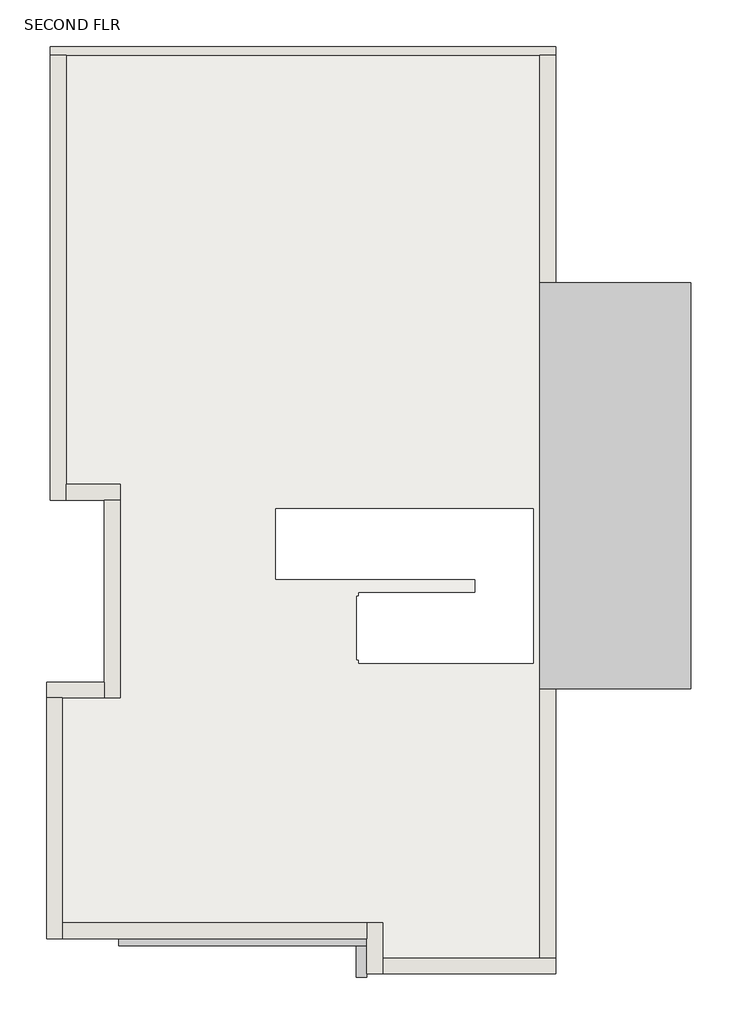
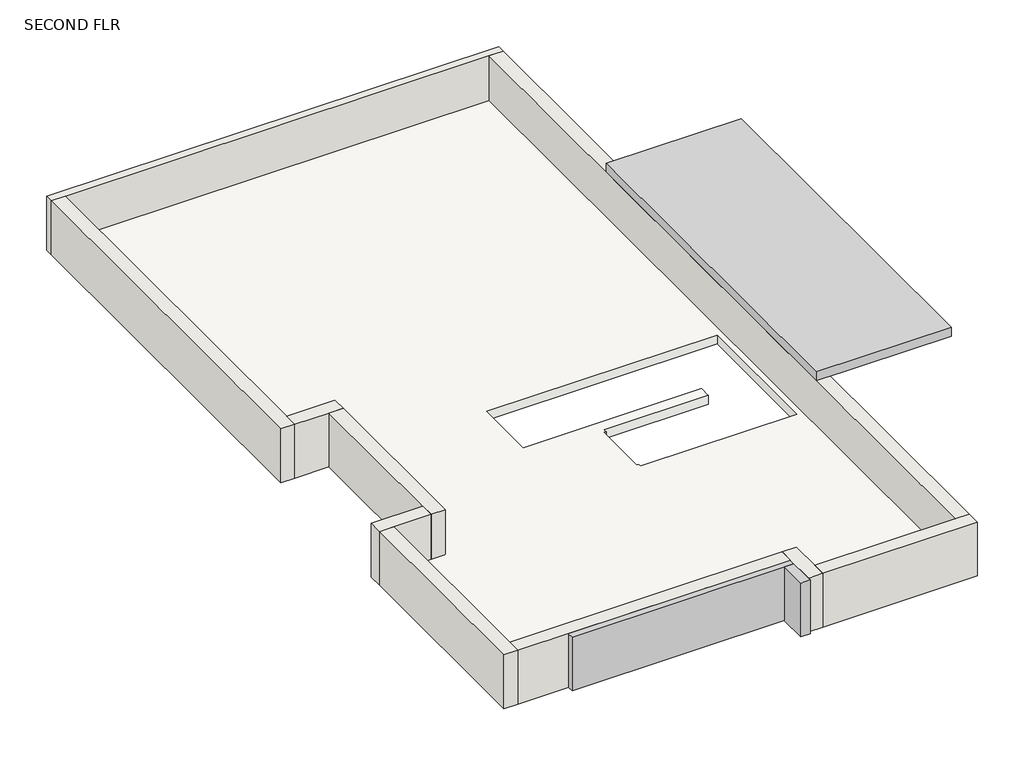
# One storey: 10 walls, 3 proxies, 1 roof.
"""IFC4 building model written with IfcOpenShell, lengths in millimetres."""

from ifc_helpers import new_model, si_unit, frame, origin, place, context, project, spatial, polyline, outline, extrude, faceted_brep, transform, mapped, element, save
from components import generic_models_10_generic_models_10_3c4deb4f, generic_models_4_generic_models_4_98a53d0d, generic_models_9_generic_models_9_5a9dd815

model = new_model("IFC4")

# Units and contexts
model_context = context("Model", 3, world=origin())
ifc_project = project(units=[si_unit("LENGTHUNIT", "METRE", prefix="MILLI")], contexts=[model_context])

# Site, building, storey
site = spatial("IfcSite", under=ifc_project)
building = spatial("IfcBuilding", under=site)
storey = spatial("IfcBuildingStorey", under=building, Name="SECOND FLR", Elevation=6096.0)

# Proxies
placement = place(None, origin())
generic_models_10_generic_models_10_shape = generic_models_10_generic_models_10_3c4deb4f(model_context)
element("IfcBuildingElementProxy", 1, Name="Generic Models 10 : Generic Models 10", ObjectType="Generic Models 10 : Generic Models 10", at=placement, inside=storey, context=model_context, shape_type="MappedRepresentation", body=[
    mapped(generic_models_10_generic_models_10_shape, transform((0.0, 0.0, 0.0), x_axis=(1.0, 0.0, 0.0), y_axis=(0.0, 1.0, 0.0), z_axis=(0.0, 0.0, 1.0))),
])
generic_models_4_generic_models_4_shape = generic_models_4_generic_models_4_98a53d0d(model_context)
element("IfcBuildingElementProxy", 2, Name="Generic Models 4 : Generic Models 4", ObjectType="Generic Models 4 : Generic Models 4", at=placement, inside=storey, context=model_context, shape_type="MappedRepresentation", body=[
    mapped(generic_models_4_generic_models_4_shape, transform((0.0, 0.0, 0.0), x_axis=(1.0, 0.0, 0.0), y_axis=(0.0, 1.0, 0.0), z_axis=(0.0, 0.0, 1.0))),
])
generic_models_9_generic_models_9_shape = generic_models_9_generic_models_9_5a9dd815(model_context)
element("IfcBuildingElementProxy", 3, Name="Generic Models 9 : Generic Models 9", ObjectType="Generic Models 9 : Generic Models 9", at=placement, inside=storey, context=model_context, shape_type="MappedRepresentation", body=[
    mapped(generic_models_9_generic_models_9_shape, transform((0.0, 0.0, 0.0), x_axis=(1.0, 0.0, 0.0), y_axis=(0.0, 1.0, 0.0), z_axis=(0.0, 0.0, 1.0))),
])

# Roof
element("IfcRoof", 4, ObjectType="FLOORING ROOF 6\"", at=placement, inside=storey, context=model_context, shape_type="SweptSolid", body=[
    extrude(outline(polyline([(-5910.1906521, 1140.4983389), (-5910.1906521, -11847.6453012), (-8170.7906521, -11847.6453012), (-8170.7906521, -11339.6453012), (-12780.8906521, -11339.6453012), (-12780.8906521, -8105.9310793), (-11952.140556, -8105.9310793), (-11952.140556, -5031.7016611), (-12726.840556, -5031.7016611), (-12726.840556, 1140.4983389), (-5910.1906521, 1140.4983389)]), holes=[polyline([(-8549.4760609, -7553.4810793), (-8517.7260609, -7553.4810793), (-8517.7260609, -7604.2810793), (-6003.1260609, -7604.2810793), (-6003.1260609, -5382.5504041), (-9709.3703437, -5382.5504041), (-9709.3703437, -6398.5504041), (-6841.3260609, -6398.5504041), (-6841.3260609, -6588.2810793), (-8517.7260609, -6588.2810793), (-8517.7260609, -6639.0810793), (-8549.4760609, -6639.0810793), (-8549.4760609, -7553.4810793)])]), frame((0.0, 0.0, 6096.0), z_axis=(0.0, 0.0, 1.0), x_axis=(1.0, 0.0, 0.0)), (0.0, 0.0, 1.0), 152.4),
])

# Walls
element("IfcWall", 5, ObjectType="EXTERIOR WALL 9\"", at=placement, inside=storey, context=model_context, shape_type="Brep", body=[
    faceted_brep([(-12955.440556, 1140.4983389, 6096.0), (-12955.440556, -5260.3016611, 6096.0), (-12955.440556, -5260.3016611, 7010.4), (-12955.440556, 1140.4983389, 7010.4), (-12726.840556, 1140.4983389, 6096.0), (-12726.840556, 1140.4983389, 7010.4), (-12726.840556, -5031.7016611, 7010.4), (-12726.840556, -5260.3016611, 7010.4), (-12726.840556, -5260.3016611, 6096.0), (-12726.840556, -5031.7016611, 6096.0)], [[[0, 1, 2, 3]], [[4, 5, 6, 7, 8, 9]], [[1, 0, 4, 9, 8]], [[3, 2, 7, 6, 5]], [[0, 3, 5, 4]], [[2, 1, 8, 7]]]),
])
element("IfcWall", 6, ObjectType="EXTERIOR WALL 9\"", at=placement, inside=storey, context=model_context, shape_type="Brep", body=[
    faceted_brep([(-12726.840556, -5260.3016611, 6096.0), (-12180.740556, -5260.3016611, 6096.0), (-11952.140556, -5260.3016611, 6096.0), (-11952.140556, -5260.3016611, 7010.4), (-12180.740556, -5260.3016611, 7010.4), (-12726.840556, -5260.3016611, 7010.4), (-12726.840556, -5031.7016611, 6096.0), (-12726.840556, -5031.7016611, 7010.4), (-11952.140556, -5031.7016611, 7010.4), (-11952.140556, -5031.7016611, 6096.0)], [[[0, 1, 2, 3, 4, 5]], [[6, 7, 8, 9]], [[2, 1, 0, 6, 9]], [[5, 4, 3, 8, 7]], [[0, 5, 7, 6]], [[3, 2, 9, 8]]]),
])
element("IfcWall", 7, ObjectType="EXTERIOR WALL 9\"", at=placement, inside=storey, context=model_context, shape_type="Brep", body=[
    faceted_brep([(-12180.740556, -5260.3016611, 6096.0), (-12180.740556, -7877.3310793, 6096.0), (-12180.740556, -8105.9310793, 6096.0), (-12180.740556, -8105.9310793, 7010.4), (-12180.740556, -7877.3310793, 7010.4), (-12180.740556, -5260.3016611, 7010.4), (-11952.140556, -5260.3016611, 6096.0), (-11952.140556, -5260.3016611, 7010.4), (-11952.140556, -8105.9310793, 7010.4), (-11952.140556, -8105.9310793, 6096.0)], [[[0, 1, 2, 3, 4, 5]], [[6, 7, 8, 9]], [[2, 1, 0, 6, 9]], [[5, 4, 3, 8, 7]], [[0, 5, 7, 6]], [[3, 2, 9, 8]]]),
])
element("IfcWall", 8, ObjectType="EXTERIOR WALL 9\"", at=placement, inside=storey, context=model_context, shape_type="Brep", body=[
    faceted_brep([(-12180.740556, -7877.3310793, 6096.0), (-13009.4906521, -7877.3310793, 6096.0), (-13009.4906521, -7877.3310793, 7010.4), (-12180.740556, -7877.3310793, 7010.4), (-12180.740556, -8105.9310793, 6096.0), (-12180.740556, -8105.9310793, 7010.4), (-12780.8906521, -8105.9310793, 7010.4), (-13009.4906521, -8105.9310793, 7010.4), (-13009.4906521, -8105.9310793, 6096.0), (-12780.8906521, -8105.9310793, 6096.0)], [[[0, 1, 2, 3]], [[4, 5, 6, 7, 8, 9]], [[1, 0, 4, 9, 8]], [[3, 2, 7, 6, 5]], [[0, 3, 5, 4]], [[2, 1, 8, 7]]]),
])
element("IfcWall", 9, ObjectType="EXTERIOR WALL 9\"", at=placement, inside=storey, context=model_context, shape_type="Brep", body=[
    faceted_brep([(-13009.4906521, -8105.9310793, 6096.0), (-13009.4906521, -11568.2453012, 6096.0), (-13009.4906521, -11568.2453012, 7010.4), (-13009.4906521, -8105.9310793, 7010.4), (-12780.8906521, -8105.9310793, 6096.0), (-12780.8906521, -8105.9310793, 7010.4), (-12780.8906521, -11339.6453012, 7010.4), (-12780.8906521, -11568.2453012, 7010.4), (-12780.8906521, -11568.2453012, 6096.0), (-12780.8906521, -11339.6453012, 6096.0)], [[[0, 1, 2, 3]], [[4, 5, 6, 7, 8, 9]], [[1, 0, 4, 9, 8]], [[3, 2, 7, 6, 5]], [[0, 3, 5, 4]], [[2, 1, 8, 7]]]),
])
element("IfcWall", 10, ObjectType="EXTERIOR WALL 9\"", at=placement, inside=storey, context=model_context, shape_type="SweptSolid", body=[
    extrude(outline(polyline([(-8399.3906521, -11568.2453012), (-12780.8906521, -11568.2453012), (-12780.8906521, -11339.6453012), (-8399.3906521, -11339.6453012), (-8399.3906521, -11568.2453012)])), frame((0.0, 0.0, 6096.0), z_axis=(0.0, 0.0, 1.0), x_axis=(1.0, 0.0, 0.0)), (0.0, 0.0, 1.0), 914.4),
])
element("IfcWall", 11, ObjectType="EXTERIOR WALL 9\"", at=placement, inside=storey, context=model_context, shape_type="Brep", body=[
    faceted_brep([(-8399.3906521, -11339.6453012, 6096.0), (-8399.3906521, -11568.2453012, 6096.0), (-8399.3906521, -12076.2453012, 6096.0), (-8399.3906521, -12076.2453012, 7010.4), (-8399.3906521, -11568.2453012, 7010.4), (-8399.3906521, -11339.6453012, 7010.4), (-8170.7906521, -11339.6453012, 6096.0), (-8170.7906521, -11339.6453012, 7010.4), (-8170.7906521, -11847.6453012, 7010.4), (-8170.7906521, -12076.2453012, 7010.4), (-8170.7906521, -12076.2453012, 6096.0), (-8170.7906521, -11847.6453012, 6096.0)], [[[0, 1, 2, 3, 4, 5]], [[6, 7, 8, 9, 10, 11]], [[2, 1, 0, 6, 11, 10]], [[5, 4, 3, 9, 8, 7]], [[0, 5, 7, 6]], [[3, 2, 10, 9]]]),
])
element("IfcWall", 12, ObjectType="EXTERIOR WALL 9\"", at=placement, inside=storey, context=model_context, shape_type="Brep", body=[
    faceted_brep([(-8170.7906521, -12076.2453012, 6096.0), (-5681.5906521, -12076.2453012, 6096.0), (-5681.5906521, -12076.2453012, 7010.4), (-8170.7906521, -12076.2453012, 7010.4), (-8170.7906521, -11847.6453012, 6096.0), (-8170.7906521, -11847.6453012, 7010.4), (-5910.1906521, -11847.6453012, 7010.4), (-5681.5906521, -11847.6453012, 7010.4), (-5681.5906521, -11847.6453012, 6096.0), (-5910.1906521, -11847.6453012, 6096.0)], [[[0, 1, 2, 3]], [[4, 5, 6, 7, 8, 9]], [[1, 0, 4, 9, 8]], [[3, 2, 7, 6, 5]], [[0, 3, 5, 4]], [[2, 1, 8, 7]]]),
])
element("IfcWall", 13, ObjectType="EXTERIOR WALL 9\"", at=placement, inside=storey, context=model_context, shape_type="SweptSolid", body=[
    extrude(outline(polyline([(-5681.5906521, 1140.4983389), (-5681.5906521, -11847.6453012), (-5910.1906521, -11847.6453012), (-5910.1906521, 1140.4983389), (-5681.5906521, 1140.4983389)])), frame((0.0, 0.0, 6096.0), z_axis=(0.0, 0.0, 1.0), x_axis=(1.0, 0.0, 0.0)), (0.0, 0.0, 1.0), 914.4),
])
element("IfcWall", 14, ObjectType="INTERIOR WALL PAINT 5\"", at=placement, inside=storey, context=model_context, shape_type="Brep", body=[
    faceted_brep([(-12955.440556, 1140.4983389, 6096.0), (-12726.840556, 1140.4983389, 6096.0), (-5910.1906521, 1140.4983389, 6096.0), (-5681.5906521, 1140.4983389, 6096.0), (-5681.5906521, 1140.4983389, 7010.4), (-5910.1906521, 1140.4983389, 7010.4), (-12726.840556, 1140.4983389, 7010.4), (-12955.440556, 1140.4983389, 7010.4), (-12955.440556, 1267.4983389, 6096.0), (-12955.440556, 1267.4983389, 7010.4), (-5681.5906521, 1267.4983389, 7010.4), (-5681.5906521, 1267.4983389, 6096.0)], [[[0, 1, 2, 3, 4, 5, 6, 7]], [[8, 9, 10, 11]], [[3, 2, 1, 0, 8, 11]], [[7, 6, 5, 4, 10, 9]], [[0, 7, 9, 8]], [[4, 3, 11, 10]]]),
])

save(model, "model.ifc")

# Revit data of these elements
# Type "FLOORING ROOF 6\""
#   Assembly Code = "B1020"
#   Layers, outside or top first: 0' - 6" "WHITE ROOFING 6\"" (function 1)
# Type "EXTERIOR WALL 9\""
#   Assembly Code = "B2010"
#   Layers, outside or top first: 0' - 9" "EXTERIOR WALL PAINT" (function 1)
# Type "INTERIOR WALL PAINT 5\""
#   Assembly Code = "B2010"
#   Layers, outside or top first: 0' - 5" "EXTERIOR WALL PAINT" (function 1)
# Element 1 (IfcBuildingElementProxy, "Generic Models 10 : Generic Models 10")
#   Phase Created = New Construction
#   Materials on its faces: "GREY COLOUR FRAME"
# Element 2 (IfcBuildingElementProxy, "Generic Models 4 : Generic Models 4")
#   Phase Created = New Construction
# Element 3 (IfcBuildingElementProxy, "Generic Models 9 : Generic Models 9")
#   Phase Created = New Construction
#   Materials on its faces: "GREY COLOUR FRAME(2)"
# Element 4 (IfcRoof, "FLOORING ROOF 6\"")
#   built-in parameter 1001705 = 20.5 (stored number, unit not read)
#   built-in parameter 1001710 = 33615
#   Phase Created = New Construction
#   Materials on its faces: "WHITE ROOFING 6\"", "MARBLE FLOORING 1'"
# Elements 5, 6, 7, 8, 9, 10, 11, 12, 13 (IfcWall, "EXTERIOR WALL 9\"")
#   Top Offset = 0' - 0"
#   Base Offset = 0' - 0"
#   Unconnected Height = 3' - 0"
#   wall height = 3' - 0"
#   Phase Created = New Construction
#   Base Constraint = SECOND FLR
#   Materials on its faces: "EXTERIOR WALL PAINT"
# Element 14 (IfcWall, "INTERIOR WALL PAINT 5\"")
#   Top Offset = 0' - 0"
#   Base Offset = 0' - 0"
#   Unconnected Height = 3' - 0"
#   wall height = 3' - 0"
#   Phase Created = New Construction
#   Base Constraint = SECOND FLR
#   Materials on its faces: "EXTERIOR WALL PAINT"
# Materials
#   "WHITE ROOFING 6\"": class "Generic", colour RGB 120 120 120, transparency 0, Cost = 0
#   "EXTERIOR WALL PAINT": class "Generic", colour RGB 120 120 120, transparency 0, Cost = 0
#   "GREY COLOUR FRAME": class "Generic", colour RGB 120 120 120, transparency 0, Cost = 0
#   "GREY COLOUR FRAME(2)": class "Generic", colour RGB 120 120 120, transparency 0, Cost = 0
#   "MARBLE FLOORING 1'": class "Generic", colour RGB 120 120 120, transparency 0, Cost = 0
